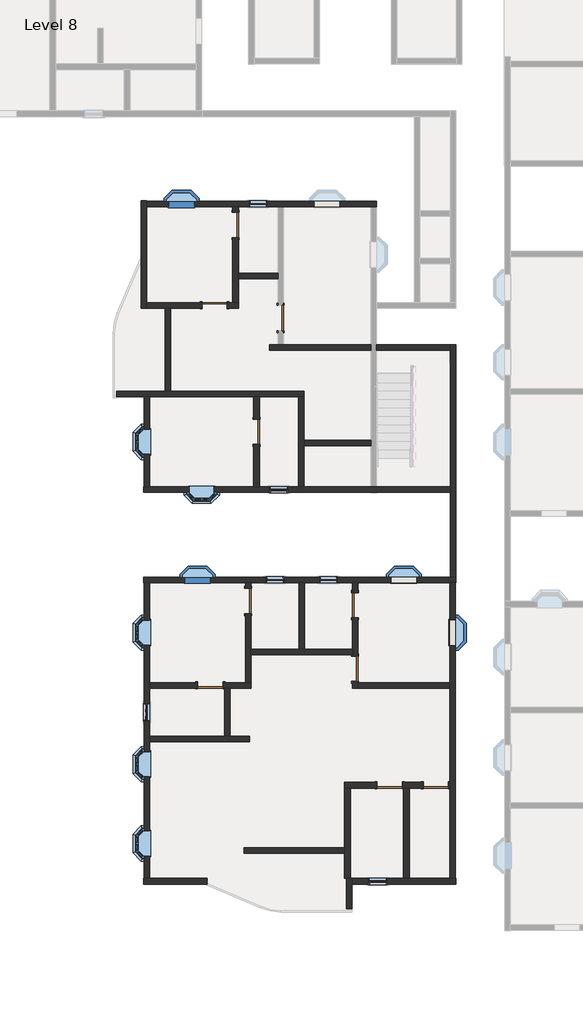
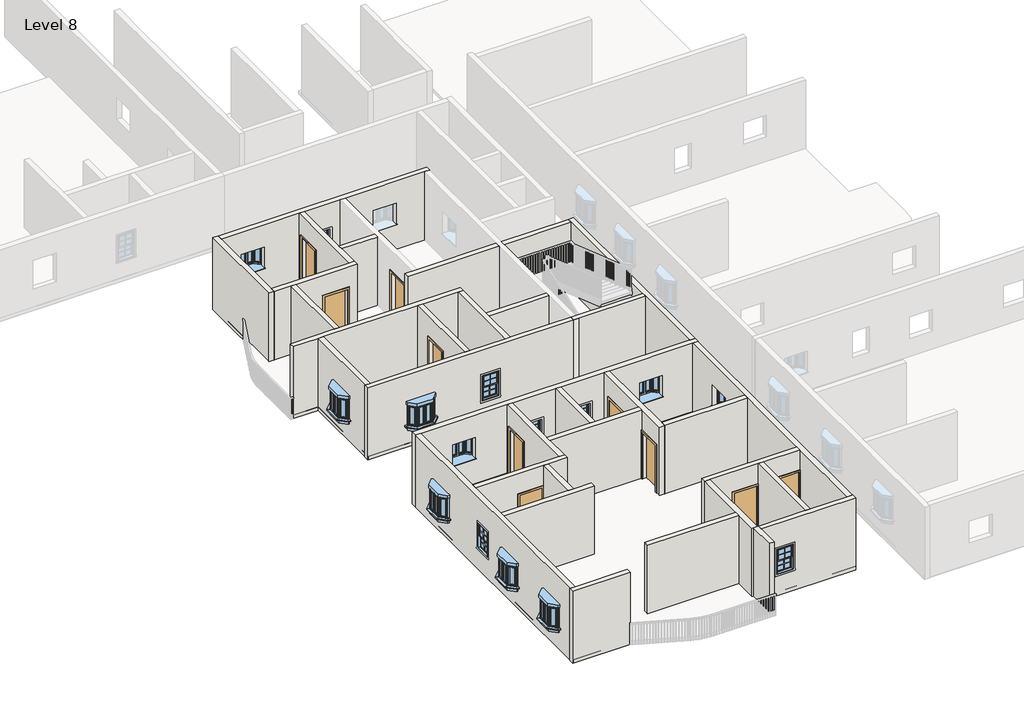
# One storey, part 1 of 14: 33 walls, 15 windows, 10 doors.
# Revit data of these elements (continued)
# Element 54 (IfcWindow, "Window-Double-Hung : 26\" x 42\"") (continued)
#   Phase Created = New Construction
#   Materials on its faces: "Wood - Stained", "Glass", "Clad - White"
# Element 55 (IfcWindow, "Window-Double-Hung : 26\" x 42\"")
#   Mark = "462"
#   Window Inset = 0' - 0"
#   Interior Wall Closure = 0' - 1 1/2"
#   Frame Extension = 0' - 1 1/4"
#   Exterior Wall Closure = 0' - 0 1/2"
#   Interior Trim Visibility = yes
#   Indicator Visibility = yes
#   Exterior Trim Visibility = yes
#   Phase Created = New Construction
#   Materials on its faces: "Wood - Stained", "Glass", "Clad - White"
# Element 56 (IfcWindow, "Window-Double-Hung : 26\" x 42\"")
#   Mark = "463"
#   Window Inset = 0' - 0"
#   Interior Wall Closure = 0' - 1 1/2"
#   Frame Extension = 0' - 1 1/4"
#   Exterior Wall Closure = 0' - 0 1/2"
#   Interior Trim Visibility = yes
#   Indicator Visibility = yes
#   Exterior Trim Visibility = yes
#   Phase Created = New Construction
#   Materials on its faces: "Wood - Stained", "Glass", "Clad - White"
# Element 57 (IfcWindow, "Window-Double-Hung : 26\" x 42\"")
#   Mark = "464"
#   Window Inset = 0' - 0"
#   Interior Wall Closure = 0' - 1 1/2"
#   Frame Extension = 0' - 1 1/4"
#   Exterior Wall Closure = 0' - 0 1/2"
#   Interior Trim Visibility = yes
#   Indicator Visibility = yes
#   Exterior Trim Visibility = yes
#   Phase Created = New Construction
#   Materials on its faces: "Wood - Stained", "Glass", "Clad - White"
# Element 58 (IfcWindow, "Window-Double-Hung : 26\" x 42\"")
#   Mark = "465"
#   Window Inset = 0' - 0"
#   Interior Wall Closure = 0' - 1 1/2"
#   Frame Extension = 0' - 1 1/4"
#   Exterior Wall Closure = 0' - 0 1/2"
#   Interior Trim Visibility = yes
#   Indicator Visibility = yes
#   Exterior Trim Visibility = yes
#   Phase Created = New Construction
#   Materials on its faces: "Wood - Stained", "Glass", "Clad - White"
# Materials
#   "Door - Panel": class "Wood", colour RGB 210 159 95, transparency 0, Cost = 0
#   "Door - Frame": colour RGB 118 70 51, transparency 0, Cost = 0
#   "Window Frame": colour RGB 249 249 249, transparency 0
#   "Glass": class "Glass", colour RGB 0 128 192, transparency 0.75, Description = "Soda Lime Glass", Cost = 0
#   "Wood - Stained": class "Wood", colour RGB 224 178 126, transparency 0, Cost = 0
#   "Clad - White": class "Wood", colour RGB 242 242 238, transparency 0, Cost = 0
#   "Default Wall": colour RGB 128 128 128, transparency 0, Cost = 0
#   "Earth": class "Generic", colour RGB 97 75 62, transparency 0, Description = "Soil", Cost = 0
#   "Parking Stripe": class "Paint", colour RGB 250 250 91, transparency 0, Cost = 0
#   "Carpet (1)": class "Carpet", colour RGB 124 80 67, transparency 0, Description = "Interior finish", Cost = 0
#   "Softwood, Lumber": class "Wood", colour RGB 223 192 134, transparency 0, Description = "Pinus Echinata", Cost = 0
